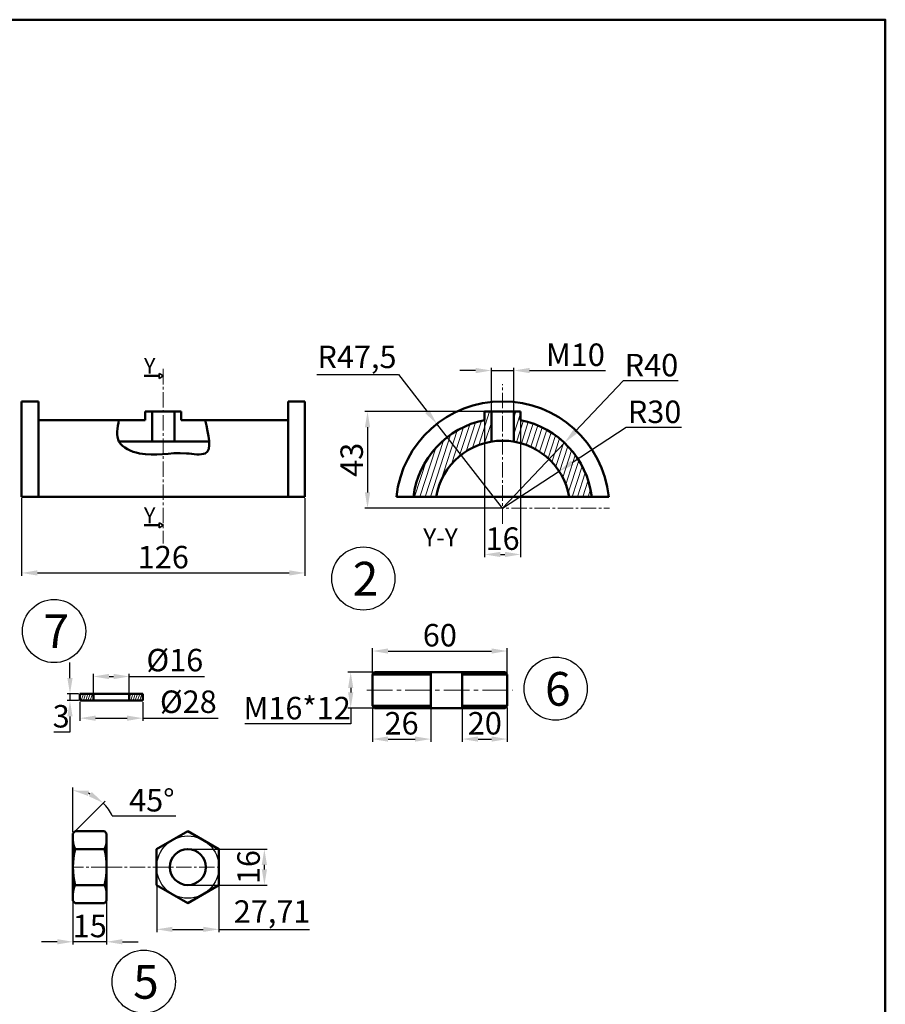
# Model space of a CAD drawing. Units: millimetres. Extents: x -68 to 1086, y -293 to 557.
# Tile 4 of 4: x 701 to 1086, y 119 to 557. Entities that reach past the tile are written whole.
import ezdxf

# ---------------------------------------------------------------- set-up
doc = ezdxf.new("R2010")
doc.units = ezdxf.units.MM
doc.header["$LTSCALE"] = 0.6
doc.linetypes.add('CENTER2', pattern=[28.575, 19.05, -3.175, 3.175, -3.175])
for name, color, linetype, lineweight in [('M-CNTR', 1, 'CENTER2', 18), ('M-DIMS', 2, 'Continuous', 25), ('M-HATC', 8, 'Continuous', 18), ('M-OUTL', 7, 'Continuous', 50), ('M-SECT', 6, 'Continuous', 35), ('M-SYMB', 4, 'Continuous', 25), ('M-TEXT', 3, 'Continuous', 25)]:
    doc.layers.add(name, color=color, linetype=linetype, lineweight=lineweight)
doc.styles.get("Standard").update_dxf_attribs({"font": 'arial.ttf'})
doc.dimstyles.new('ISO-25', dxfattribs={"dimtxt": 10, "dimasz": 7, "dimexe": 1.25, "dimexo": 0.625, "dimtad": 1, "dimtoh": 1, "dimtxsty": 'Standard', "dimcen": 2.5, "dimadec": 0, "dimazin": 0, "dimtfac": 1, "dimtmove": 0, "dimatfit": 3, "dimfxl": 1, "dimarcsym": 0})

# ---------------------------------------------------------------- blocks, each defined once
blk = doc.blocks.new('*D54')
at = {"layer": 'Defpoints', "color": 0, "ltscale": 0.6, "transparency": 16777216}
for p in [(701.62, 344.28), (827.62, 344.28), (827.62, 310.45)]:
    blk.add_point(p, dxfattribs=at)
at = {"layer": 'M-DIMS', "color": 0, "lineweight": -2, "ltscale": 0.6, "transparency": 16777216}
for p, q in [((701.62, 343.66), (701.62, 309.2)), ((827.62, 343.66), (827.62, 309.2)), ((708.62, 310.45), (820.62, 310.45))]:
    blk.add_line(p, q, dxfattribs=at)
at = {"layer": 'M-DIMS', "color": 0, "ltscale": 0.6, "transparency": 16777216}
for points in [[(708.62, 311.62), (708.62, 309.28), (701.62, 310.45)], [(820.62, 311.62), (820.62, 309.28), (827.62, 310.45)]]:
    blk.add_solid(points, dxfattribs=at)
at = {"layer": 'M-DIMS', "color": 0, "ltscale": 0.6, "transparency": 16777216, "insert": (764.62, 316.18), "char_height": 10, "attachment_point": 5}
blk.add_mtext('126', dxfattribs=at)
blk = doc.blocks.new('*D55')
at = {"layer": 'Defpoints', "color": 0, "ltscale": 0.6, "transparency": 16777216}
for p in [(940.63, 355.65), (915.49, 339.28)]:
    blk.add_point(p, dxfattribs=at)
at = {"layer": 'M-DIMS', "color": 0, "lineweight": -2, "ltscale": 0.6, "transparency": 16777216}
for p, q in [((970.51, 375.11), (946.5, 359.47)), ((995, 375.11), (970.51, 375.11)), ((915.49, 339.28), (940.63, 355.65))]:
    blk.add_line(p, q, dxfattribs=at)
at = {"layer": 'M-DIMS', "color": 0, "ltscale": 0.6, "transparency": 16777216}
blk.add_solid([(945.86, 360.45), (947.13, 358.5), (940.63, 355.65)], dxfattribs=at)
at = {"layer": 'M-DIMS', "color": 0, "ltscale": 0.6, "transparency": 16777216, "insert": (983.07, 380.84), "char_height": 10, "attachment_point": 5}
blk.add_mtext('R30', dxfattribs=at)
blk = doc.blocks.new('*D56')
at = {"layer": 'Defpoints', "color": 0, "ltscale": 0.6, "transparency": 16777216}
for p in [(943, 368.32), (915.49, 339.28)]:
    blk.add_point(p, dxfattribs=at)
at = {"layer": 'M-DIMS', "color": 0, "lineweight": -2, "ltscale": 0.6, "transparency": 16777216}
for p, q in [((969.12, 395.89), (947.82, 373.4)), ((993.61, 395.89), (969.12, 395.89)), ((915.49, 339.28), (943, 368.32))]:
    blk.add_line(p, q, dxfattribs=at)
at = {"layer": 'M-DIMS', "color": 0, "ltscale": 0.6, "transparency": 16777216}
blk.add_solid([(946.97, 374.21), (948.66, 372.6), (943, 368.32)], dxfattribs=at)
at = {"layer": 'M-DIMS', "color": 0, "ltscale": 0.6, "transparency": 16777216, "insert": (981.68, 401.62), "char_height": 10, "attachment_point": 5}
blk.add_mtext('R40', dxfattribs=at)
blk = doc.blocks.new('*D57')
at = {"layer": 'Defpoints', "color": 0, "ltscale": 0.6, "transparency": 16777216}
for p in [(886.28, 376.74), (915.49, 339.28)]:
    blk.add_point(p, dxfattribs=at)
at = {"layer": 'M-DIMS', "color": 0, "lineweight": -2, "ltscale": 0.6, "transparency": 16777216}
for p, q in [((832.92, 398.68), (869.17, 398.68)), ((869.17, 398.68), (881.97, 382.26)), ((915.49, 339.28), (886.28, 376.74))]:
    blk.add_line(p, q, dxfattribs=at)
at = {"layer": 'M-DIMS', "color": 0, "ltscale": 0.6, "transparency": 16777216}
blk.add_solid([(882.89, 382.98), (881.05, 381.54), (886.28, 376.74)], dxfattribs=at)
at = {"layer": 'M-DIMS', "color": 0, "ltscale": 0.6, "transparency": 16777216, "insert": (850.73, 405.29), "char_height": 10, "attachment_point": 5}
blk.add_mtext('R47,5', dxfattribs=at)
blk = doc.blocks.new('*D58')
at = {"layer": 'Defpoints', "color": 0, "ltscale": 0.6, "transparency": 16777216}
for p in [(907.49, 382.28), (923.49, 382.28), (923.49, 318.67)]:
    blk.add_point(p, dxfattribs=at)
at = {"layer": 'M-DIMS', "color": 0, "lineweight": -2, "ltscale": 0.6, "transparency": 16777216}
for p, q in [((907.49, 381.66), (907.49, 317.42)), ((923.49, 381.66), (923.49, 317.42)), ((914.49, 318.67), (916.49, 318.67))]:
    blk.add_line(p, q, dxfattribs=at)
at = {"layer": 'M-DIMS', "color": 0, "ltscale": 0.6, "transparency": 16777216}
for points in [[(914.49, 319.84), (914.49, 317.51), (907.49, 318.67)], [(916.49, 319.84), (916.49, 317.51), (923.49, 318.67)]]:
    blk.add_solid(points, dxfattribs=at)
at = {"layer": 'M-DIMS', "color": 0, "ltscale": 0.6, "transparency": 16777216, "insert": (915.49, 324.41), "char_height": 10, "attachment_point": 5}
blk.add_mtext('16', dxfattribs=at)
blk = doc.blocks.new('*D59')
at = {"layer": 'Defpoints', "color": 0, "ltscale": 0.6, "transparency": 16777216}
for p in [(920.49, 400.5), (910.49, 382.28), (920.49, 382.28)]:
    blk.add_point(p, dxfattribs=at)
at = {"layer": 'M-DIMS', "color": 0, "lineweight": -2, "ltscale": 0.6, "transparency": 16777216}
for p, q in [((903.49, 400.5), (896.49, 400.5)), ((910.49, 382.91), (910.49, 401.75)), ((910.49, 400.5), (920.49, 400.5)), ((920.49, 382.91), (920.49, 401.75)), ((927.49, 400.5), (961.21, 400.5))]:
    blk.add_line(p, q, dxfattribs=at)
at = {"layer": 'M-DIMS', "color": 0, "ltscale": 0.6, "transparency": 16777216}
for points in [[(903.49, 401.66), (903.49, 399.33), (910.49, 400.5)], [(927.49, 401.66), (927.49, 399.33), (920.49, 400.5)]]:
    blk.add_solid(points, dxfattribs=at)
at = {"layer": 'M-DIMS', "color": 0, "ltscale": 0.6, "transparency": 16777216, "insert": (947.85, 406.23), "char_height": 10, "attachment_point": 5}
blk.add_mtext('M10', dxfattribs=at)
blk = doc.blocks.new('*D60')
at = {"layer": 'Defpoints', "color": 0, "ltscale": 0.6, "transparency": 16777216}
for p in [(915.49, 382.28), (855.42, 339.28), (915.49, 339.28)]:
    blk.add_point(p, dxfattribs=at)
at = {"layer": 'M-DIMS', "color": 0, "lineweight": -2, "ltscale": 0.6, "transparency": 16777216}
for p, q in [((914.87, 382.28), (854.17, 382.28)), ((855.42, 375.28), (855.42, 346.28)), ((914.87, 339.28), (854.17, 339.28))]:
    blk.add_line(p, q, dxfattribs=at)
at = {"layer": 'M-DIMS', "color": 0, "ltscale": 0.6, "transparency": 16777216}
for points in [[(854.26, 375.28), (856.59, 375.28), (855.42, 382.28)], [(854.26, 346.28), (856.59, 346.28), (855.42, 339.28)]]:
    blk.add_solid(points, dxfattribs=at)
at = {"layer": 'M-DIMS', "color": 0, "ltscale": 0.6, "transparency": 16777216, "insert": (849.69, 360.78), "char_height": 10, "attachment_point": 5, "rotation": 90}
blk.add_mtext('43', dxfattribs=at)
blk = doc.blocks.new('*D61')
at = {"layer": 'Defpoints', "color": 0, "ltscale": 0.6, "transparency": 16777216}
for p in [(749.5, 264.36), (733.5, 256.64), (749.5, 256.64)]:
    blk.add_point(p, dxfattribs=at)
at = {"layer": 'M-DIMS', "color": 0, "lineweight": -2, "ltscale": 0.6, "transparency": 16777216}
for p, q in [((733.5, 257.26), (733.5, 265.61)), ((740.5, 264.36), (742.5, 264.36)), ((749.5, 257.26), (749.5, 265.61)), ((749.5, 264.36), (782.95, 264.36))]:
    blk.add_line(p, q, dxfattribs=at)
at = {"layer": 'M-DIMS', "color": 0, "ltscale": 0.6, "transparency": 16777216}
for points in [[(740.5, 265.53), (740.5, 263.19), (733.5, 264.36)], [(742.5, 265.53), (742.5, 263.19), (749.5, 264.36)]]:
    blk.add_solid(points, dxfattribs=at)
at = {"layer": 'M-DIMS', "color": 0, "ltscale": 0.6, "transparency": 16777216, "insert": (769.73, 270.37), "char_height": 10, "attachment_point": 5}
blk.add_mtext('%%C16', dxfattribs=at)
blk = doc.blocks.new('*D62')
at = {"layer": 'Defpoints', "color": 0, "ltscale": 0.6, "transparency": 16777216}
for p in [(727.5, 253.64), (755.5, 253.64), (755.5, 245.83)]:
    blk.add_point(p, dxfattribs=at)
at = {"layer": 'M-DIMS', "color": 0, "lineweight": -2, "ltscale": 0.6, "transparency": 16777216}
for p, q in [((727.5, 253.01), (727.5, 244.58)), ((755.5, 253.01), (755.5, 244.58)), ((734.5, 245.83), (748.5, 245.83)), ((755.5, 245.83), (788.98, 245.83))]:
    blk.add_line(p, q, dxfattribs=at)
at = {"layer": 'M-DIMS', "color": 0, "ltscale": 0.6, "transparency": 16777216}
for points in [[(734.5, 246.99), (734.5, 244.66), (727.5, 245.83)], [(748.5, 246.99), (748.5, 244.66), (755.5, 245.83)]]:
    blk.add_solid(points, dxfattribs=at)
at = {"layer": 'M-DIMS', "color": 0, "ltscale": 0.6, "transparency": 16777216, "insert": (775.74, 251.84), "char_height": 10, "attachment_point": 5}
blk.add_mtext('%%C28', dxfattribs=at)
blk = doc.blocks.new('*D63')
at = {"layer": 'Defpoints', "color": 0, "ltscale": 0.6, "transparency": 16777216}
for p in [(727.5, 256.64), (723.1, 253.64), (727.5, 253.64)]:
    blk.add_point(p, dxfattribs=at)
at = {"layer": 'M-DIMS', "color": 0, "lineweight": -2, "ltscale": 0.6, "transparency": 16777216}
for p, q in [((723.1, 263.64), (723.1, 270.64)), ((726.88, 256.64), (721.85, 256.64)), ((723.1, 256.64), (723.1, 253.64)), ((726.88, 253.64), (721.85, 253.64)), ((723.1, 246.64), (723.1, 239.64)), ((723.1, 239.64), (715.93, 239.64))]:
    blk.add_line(p, q, dxfattribs=at)
at = {"layer": 'M-DIMS', "color": 0, "ltscale": 0.6, "transparency": 16777216}
for points in [[(721.94, 263.64), (724.27, 263.64), (723.1, 256.64)], [(721.94, 246.64), (724.27, 246.64), (723.1, 253.64)]]:
    blk.add_solid(points, dxfattribs=at)
at = {"layer": 'M-DIMS', "color": 0, "ltscale": 0.6, "transparency": 16777216, "insert": (719.2, 245.37), "char_height": 10, "attachment_point": 5}
blk.add_mtext('3', dxfattribs=at)
blk = doc.blocks.new('*D64')
at = {"layer": 'Defpoints', "color": 0, "ltscale": 0.6, "transparency": 16777216}
for p in [(724.42, 166.01), (739.42, 166.01), (724.42, 146.34)]:
    blk.add_point(p, dxfattribs=at)
at = {"layer": 'M-DIMS', "color": 0, "lineweight": -2, "ltscale": 0.6, "transparency": 16777216}
for p, q in [((724.42, 165.39), (724.42, 145.09)), ((739.42, 165.39), (739.42, 145.09)), ((717.42, 146.34), (710.42, 146.34)), ((739.42, 146.34), (724.42, 146.34)), ((746.42, 146.34), (753.42, 146.34))]:
    blk.add_line(p, q, dxfattribs=at)
at = {"layer": 'M-DIMS', "color": 0, "ltscale": 0.6, "transparency": 16777216}
for points in [[(717.42, 147.51), (717.42, 145.17), (724.42, 146.34)], [(746.42, 147.51), (746.42, 145.17), (739.42, 146.34)]]:
    blk.add_solid(points, dxfattribs=at)
at = {"layer": 'M-DIMS', "color": 0, "ltscale": 0.6, "transparency": 16777216, "insert": (731.92, 152.07), "char_height": 10, "attachment_point": 5}
blk.add_mtext('15', dxfattribs=at)
blk = doc.blocks.new('*D65')
at = {"layer": 'Defpoints', "color": 0, "ltscale": 0.6, "transparency": 16777216}
for p in [(729.37, 213.02), (724.42, 194.57), (724.42, 194.57), (725.42, 195.57), (724.42, 164.57)]:
    blk.add_point(p, dxfattribs=at)
at = {"layer": 'M-DIMS', "color": 0, "lineweight": -2, "ltscale": 0.6, "transparency": 16777216}
for p, q in [((724.42, 195.2), (724.42, 214.93)), ((725.87, 196.02), (738.81, 208.96)), ((741.89, 202.31), (770.16, 202.31))]:
    blk.add_line(p, q, dxfattribs=at)
for start, end in [(66.1169, 68.8831), (23.8831, 45)]:
    blk.add_arc((724.42, 194.57), 19.1, start, end, dxfattribs=at)
at = {"layer": 'M-DIMS', "color": 0, "ltscale": 0.6, "transparency": 16777216}
for points in [[(731.09, 211.25), (731.52, 213.54), (724.42, 213.68)], [(732.82, 213), (731.5, 211.08), (737.93, 208.08)]]:
    blk.add_solid(points, dxfattribs=at)
at = {"layer": 'M-DIMS', "color": 0, "ltscale": 0.6, "transparency": 16777216, "insert": (759.52, 208.02), "char_height": 10, "attachment_point": 5}
blk.add_mtext('45°', dxfattribs=at)
blk = doc.blocks.new('*D66')
at = {"layer": 'Defpoints', "color": 0, "ltscale": 0.6, "transparency": 16777216}
for p in [(761.66, 171.57), (789.37, 171.57), (789.37, 151.87)]:
    blk.add_point(p, dxfattribs=at)
at = {"layer": 'M-DIMS', "color": 0, "lineweight": -2, "ltscale": 0.6, "transparency": 16777216}
for p, q in [((761.66, 170.95), (761.66, 150.62)), ((789.37, 170.95), (789.37, 150.62)), ((768.66, 151.87), (782.37, 151.87)), ((789.37, 151.87), (829.6, 151.87))]:
    blk.add_line(p, q, dxfattribs=at)
at = {"layer": 'M-DIMS', "color": 0, "ltscale": 0.6, "transparency": 16777216}
for points in [[(768.66, 153.03), (768.66, 150.7), (761.66, 151.87)], [(782.37, 153.03), (782.37, 150.7), (789.37, 151.87)]]:
    blk.add_solid(points, dxfattribs=at)
at = {"layer": 'M-DIMS', "color": 0, "ltscale": 0.6, "transparency": 16777216, "insert": (812.99, 158.5), "char_height": 10, "attachment_point": 5}
blk.add_mtext('27,71', dxfattribs=at)
blk = doc.blocks.new('*D67')
at = {"layer": 'Defpoints', "color": 0, "ltscale": 0.6, "transparency": 16777216}
for p in [(775.51, 187.57), (809.56, 187.57), (775.51, 171.57)]:
    blk.add_point(p, dxfattribs=at)
at = {"layer": 'M-DIMS', "color": 0, "lineweight": -2, "ltscale": 0.6, "transparency": 16777216}
for p, q in [((776.14, 187.57), (810.81, 187.57)), ((809.56, 178.57), (809.56, 180.57)), ((776.14, 171.57), (810.81, 171.57))]:
    blk.add_line(p, q, dxfattribs=at)
at = {"layer": 'M-DIMS', "color": 0, "ltscale": 0.6, "transparency": 16777216}
for points in [[(808.39, 180.57), (810.72, 180.57), (809.56, 187.57)], [(808.39, 178.57), (810.72, 178.57), (809.56, 171.57)]]:
    blk.add_solid(points, dxfattribs=at)
at = {"layer": 'M-DIMS', "color": 0, "ltscale": 0.6, "transparency": 16777216, "insert": (803.83, 179.57), "char_height": 10, "attachment_point": 5, "rotation": 90}
blk.add_mtext('16', dxfattribs=at)
blk = doc.blocks.new('*U71')
at = {"layer": 'M-CNTR', "color": 0, "transparency": 16777216}
blk.add_line((-32.5, 0), (32.5, 0), dxfattribs=at)
blk = doc.blocks.new('*D72')
at = {"layer": 'Defpoints', "color": 0, "ltscale": 0.6, "transparency": 16777216}
for p in [(917.58, 275.7), (857.58, 262.16), (917.58, 262.16)]:
    blk.add_point(p, dxfattribs=at)
at = {"layer": 'M-DIMS', "color": 0, "lineweight": -2, "ltscale": 0.6, "transparency": 16777216}
for p, q in [((857.58, 262.78), (857.58, 276.95)), ((917.58, 262.78), (917.58, 276.95)), ((864.58, 275.7), (910.58, 275.7))]:
    blk.add_line(p, q, dxfattribs=at)
at = {"layer": 'M-DIMS', "color": 0, "ltscale": 0.6, "transparency": 16777216}
for points in [[(864.58, 276.87), (864.58, 274.54), (857.58, 275.7)], [(910.58, 276.87), (910.58, 274.54), (917.58, 275.7)]]:
    blk.add_solid(points, dxfattribs=at)
at = {"layer": 'M-DIMS', "color": 0, "ltscale": 0.6, "transparency": 16777216, "insert": (887.58, 281.43), "char_height": 10, "attachment_point": 5}
blk.add_mtext('60', dxfattribs=at)
blk = doc.blocks.new('*D73')
at = {"layer": 'Defpoints', "color": 0, "ltscale": 0.6, "transparency": 16777216}
for p in [(857.58, 251.27), (883.58, 251.27), (883.58, 236.53)]:
    blk.add_point(p, dxfattribs=at)
at = {"layer": 'M-DIMS', "color": 0, "lineweight": -2, "ltscale": 0.6, "transparency": 16777216}
for p, q in [((857.58, 250.64), (857.58, 235.28)), ((883.58, 250.64), (883.58, 235.28)), ((864.58, 236.53), (876.58, 236.53))]:
    blk.add_line(p, q, dxfattribs=at)
at = {"layer": 'M-DIMS', "color": 0, "ltscale": 0.6, "transparency": 16777216}
for points in [[(864.58, 237.7), (864.58, 235.37), (857.58, 236.53)], [(876.58, 237.7), (876.58, 235.37), (883.58, 236.53)]]:
    blk.add_solid(points, dxfattribs=at)
at = {"layer": 'M-DIMS', "color": 0, "ltscale": 0.6, "transparency": 16777216, "insert": (870.58, 242.26), "char_height": 10, "attachment_point": 5}
blk.add_mtext('26', dxfattribs=at)
blk = doc.blocks.new('*D74')
at = {"layer": 'Defpoints', "color": 0, "ltscale": 0.6, "transparency": 16777216}
for p in [(897.58, 251.27), (917.58, 251.27), (917.58, 236.53)]:
    blk.add_point(p, dxfattribs=at)
at = {"layer": 'M-DIMS', "color": 0, "lineweight": -2, "ltscale": 0.6, "transparency": 16777216}
for p, q in [((897.58, 250.64), (897.58, 235.28)), ((917.58, 250.64), (917.58, 235.28)), ((904.58, 236.53), (910.58, 236.53))]:
    blk.add_line(p, q, dxfattribs=at)
at = {"layer": 'M-DIMS', "color": 0, "ltscale": 0.6, "transparency": 16777216}
for points in [[(904.58, 237.7), (904.58, 235.37), (897.58, 236.53)], [(910.58, 237.7), (910.58, 235.37), (917.58, 236.53)]]:
    blk.add_solid(points, dxfattribs=at)
at = {"layer": 'M-DIMS', "color": 0, "ltscale": 0.6, "transparency": 16777216, "insert": (907.58, 242.26), "char_height": 10, "attachment_point": 5}
blk.add_mtext('20', dxfattribs=at)
blk = doc.blocks.new('*D75')
at = {"layer": 'Defpoints', "color": 0, "ltscale": 0.6, "transparency": 16777216}
for p in [(858.58, 266.27), (847.94, 250.27), (858.58, 250.27)]:
    blk.add_point(p, dxfattribs=at)
at = {"layer": 'M-DIMS', "color": 0, "lineweight": -2, "ltscale": 0.6, "transparency": 16777216}
for p, q in [((857.95, 266.27), (846.69, 266.27)), ((847.94, 259.27), (847.94, 257.27)), ((857.95, 250.27), (846.69, 250.27)), ((847.94, 250.27), (847.94, 243.27)), ((847.94, 243.27), (800.93, 243.27))]:
    blk.add_line(p, q, dxfattribs=at)
at = {"layer": 'M-DIMS', "color": 0, "ltscale": 0.6, "transparency": 16777216}
for points in [[(846.77, 259.27), (849.1, 259.27), (847.94, 266.27)], [(846.77, 257.27), (849.1, 257.27), (847.94, 250.27)]]:
    blk.add_solid(points, dxfattribs=at)
at = {"layer": 'M-DIMS', "color": 0, "ltscale": 0.6, "transparency": 16777216, "insert": (824.12, 249), "char_height": 10, "attachment_point": 5}
blk.add_mtext('M16*12', dxfattribs=at)
blk = doc.blocks.new('NUT-SIDE')
at = {"ltscale": 0.6}
for p, q in [((1, 32), (0, 31)), ((0, 1), (0, 31)), ((1, 32), (14, 32)), ((15, 31), (14, 32)), ((15, 31), (15, 1)), ((14, 24), (1, 24)), ((14, 8), (1, 8)), ((0, 1), (1, 0)), ((14, 0), (1, 0)), ((15, 1), (14, 0))]:
    blk.add_line(p, q, dxfattribs=at)
for centre, radius, start, end in [((8.5, 28), 8.5, 180, 208.0725), ((6.5, 28), 8.5, 331.9275, 0), ((32.5, 16), 32.5, 165.75, 194.25), ((-17.5, 16), 32.5, 345.75, 14.25), ((8.5, 4), 8.5, 151.9275, 180), ((6.5, 4), 8.5, 0, 28.0725)]:
    blk.add_arc(centre, radius, start, end, dxfattribs=at)
blk = doc.blocks.new('WASHER-SIDE')
at = {"ltscale": 0.6}
for p, q in [((0, 3), (28, 3)), ((0, 0), (0, 3)), ((28, 0), (0, 0)), ((28, 3), (28, 0))]:
    blk.add_line(p, q, dxfattribs=at)
blk = doc.blocks.new('SECT-ARROW')
at = {"ltscale": 0.6}
for p, q in [((1.92, 1.11), (0, 2.22)), ((0, 2.22), (0, 0)), ((1.92, 1.11), (0, 0))]:
    blk.add_line(p, q, dxfattribs=at)

msp = doc.modelspace()

# ---------------------------------------------------------------- hatches: boundary and pattern name
at = {"layer": 'M-HATC', "ltscale": 0.6}
h = msp.add_hatch(dxfattribs=at)
h.set_pattern_fill('ANSI31', color=256, scale=0.7, angle=27)
h.set_pattern_definition([(72, (166.6146, 303.1702), (-2.113723, 0.68679), [])])
h.paths.add_polyline_path([(910.492, 368.865), (910.492, 382.284), (907.492, 382.284), (907.492, 378.476, 0.321461), (875.805, 344.284), (885.911, 344.284, -0.3191977)])
h.paths.add_polyline_path([(945.072, 344.284), (955.178, 344.284, 0.321461), (923.492, 378.476), (923.492, 382.284), (920.492, 382.284), (920.492, 368.865, -0.3191977)])
h = msp.add_hatch(dxfattribs=at)
h.set_pattern_fill('ANSI31', color=256, scale=0.3, angle=27)
h.set_pattern_definition([(72, (-83.0523, 25.7486), (-0.9058813, 0.2943387), [])])
h.paths.add_polyline_path([(749.502, 256.636), (749.502, 253.636), (755.502, 253.636), (755.502, 256.636)])
h.paths.add_polyline_path([(733.502, 253.636), (733.502, 256.636), (727.502, 256.636), (727.502, 253.636)])

# ---------------------------------------------------------------- linework, layer by layer
at = {"layer": 'M-CNTR', "ltscale": 0.6}
for p, q in [((764.618, 401.189), (764.618, 323.467)), ((915.492, 332.296), (915.492, 394.447)), ((867.992, 339.284), (962.992, 339.284)), ((739.424, 179.574), (724.424, 179.574)), ((739.424, 179.574), (790.587, 179.574))]:
    msp.add_line(p, q, dxfattribs=at)
at = {"layer": 'M-OUTL', "ltscale": 0.6}
for p, q in [((762.886, 398.105), (756.143, 398.105)), ((701.618, 344.284), (701.618, 386.784)), ((701.618, 386.784), (709.118, 386.784)), ((709.118, 386.784), (709.118, 344.284)), ((820.118, 386.784), (820.118, 344.284)), ((820.118, 386.784), (827.618, 386.784)), ((827.618, 344.284), (827.618, 386.784)), ((772.618, 382.284), (756.618, 382.284)), ((756.618, 382.284), (756.618, 378.476)), ((759.618, 382.284), (759.618, 368.865)), ((769.618, 382.284), (769.618, 368.865)), ((772.618, 382.284), (772.618, 378.476)), ((907.492, 378.476), (907.492, 382.284)), ((907.492, 382.284), (923.492, 382.284)), ((910.492, 368.865), (910.492, 382.284)), ((920.492, 368.865), (920.492, 382.284)), ((923.492, 378.476), (923.492, 382.284)), ((756.618, 378.476), (709.118, 378.476)), ((820.118, 378.476), (772.618, 378.476)), ((785.053, 368.865), (744.907, 368.865)), ((827.618, 344.284), (701.618, 344.284)), ((868.255, 344.284), (962.728, 344.284)), ((762.886, 331.637), (756.143, 331.637)), ((858.577, 266.27), (857.577, 265.27)), ((857.577, 251.27), (857.577, 265.27)), ((857.577, 265.27), (883.577, 265.27)), ((858.577, 266.27), (916.577, 266.27)), ((883.577, 250.27), (883.577, 266.27)), ((897.577, 266.27), (897.577, 250.27)), ((917.577, 265.27), (897.577, 265.27)), ((916.577, 266.27), (917.577, 265.27)), ((917.577, 265.27), (917.577, 251.27)), ((733.502, 253.636), (733.502, 256.636)), ((749.502, 256.636), (749.502, 253.636)), ((857.577, 251.27), (858.577, 250.27)), ((857.577, 251.27), (883.577, 251.27)), ((916.577, 250.27), (858.577, 250.27)), ((917.577, 251.27), (897.577, 251.27)), ((917.577, 251.27), (916.577, 250.27))]:
    msp.add_line(p, q, dxfattribs=at)
for points in [[(-68.392, 556.589), (1085.677, 556.589), (1085.677, -292.72), (-68.392, -292.72)], [(775.512, 195.574), (761.656, 187.574), (761.656, 171.574), (775.512, 163.574), (789.369, 171.574), (789.369, 187.574)]]:
    msp.add_lwpolyline(points, close=True, dxfattribs=at)
msp.add_circle((775.512, 179.574), 8, dxfattribs=at)
for radius, start, end in [(47.5, 6.04233, 173.95767), (40, 101.53696, 172.81924), (40, 7.18076, 78.46304), (30, 9.59407, 170.40593)]:
    msp.add_arc((915.492, 339.284), radius, start, end, dxfattribs=at)
msp.add_open_spline([(744.907, 378.476), (744.219, 374.956), (742.781, 367.601), (758.245, 361.048), (769.461, 365.066), (787.388, 361.544), (784.827, 371.858), (783.183, 378.476)], degree=3, knots=[0, 0, 0, 0, 9.611437, 20.0803576, 40.9991508, 49.2899789, 64.1358762, 64.1358762, 64.1358762, 64.1358762], dxfattribs=at)
at = {"layer": 'M-SYMB', "ltscale": 0.6}
for centre, radius in [((853.555, 307.967), 14.053), ((716.05, 284.583), 14.053), ((939.076, 258.962), 14.053), ((775.512, 179.574), 13.856), ((755.919, 128.606), 14.053)]:
    msp.add_circle(centre, radius, dxfattribs=at)

# ---------------------------------------------------------------- block references
at = {"layer": 'M-CNTR'}
msp.add_blockref('*U71', (887.577, 258.27), dxfattribs=at)
at = {"layer": 'M-OUTL'}
for name, p in [('WASHER-SIDE', (727.502, 253.636)), ('NUT-SIDE', (724.424, 163.574))]:
    msp.add_blockref(name, p, dxfattribs=at)
at = {"layer": 'M-SECT'}
for p in [(762.824, 396.996), (762.824, 330.529)]:
    msp.add_blockref('SECT-ARROW', p, dxfattribs=at)

# ---------------------------------------------------------------- texts
at = {"layer": 'M-TEXT', "ltscale": 0.6, "attachment_point": 1}
for s, width, insert, char_height in [('Y', 4.24472, (756.023, 406.049), 7), ('Y', 4.24472, (756.023, 339.582), 7), ('Y-Y', 23.26032, (880.17, 330.264), 8), ('2', 15, (848.849, 315.374), 15), ('7', 15, (711.344, 291.99), 15), ('6', 15, (934.37, 266.369), 15), ('5', 15, (751.213, 136.013), 15)]:
    msp.add_mtext_dynamic_manual_height_columns(s, width=width, gutter_width=12.5, heights=[0], dxfattribs=dict(at, insert=insert, char_height=char_height))

# ---------------------------------------------------------------- dimensions: what is measured, and where the dimension line sits
at = {"layer": 'M-DIMS', "ltscale": 0.6}
for mpoint, picture, middle in [((886.279, 376.739), '*D57', (850.732, 398.679)), ((943.002, 368.322), '*D56', (981.675, 395.889)), ((940.632, 355.654), '*D55', (983.068, 375.11))]:
    dim = msp.add_radius_dim(center=(915.492, 339.284), mpoint=mpoint, dimstyle='ISO-25', override={"dimclrd": 0, "dimclre": 0, "dimclrt": 0}, dxfattribs=at)
    dim.commit()
    dim.dimension.update_dxf_attribs({"geometry": picture, "text_midpoint": middle, "dimtype": 164})
for base, p1, p2, text, picture, middle in [((920.492, 400.495), (910.492, 382.284), (920.492, 382.284), 'M<>', '*D59', (947.852, 406.226)), ((749.502, 264.361), (733.502, 256.636), (749.502, 256.636), '%%C<>', '*D61', (769.726, 270.371))]:
    dim = msp.add_linear_dim(base=base, p1=p1, p2=p2, text=text, dimstyle='ISO-25', override={"dimclrd": 0, "dimclre": 0, "dimclrt": 0}, dxfattribs=at)
    dim.commit()
    dim.dimension.update_dxf_attribs({"geometry": picture, "text_midpoint": middle})
for base, p1, p2, picture, middle in [((855.424, 339.284), (915.492, 382.284), (915.492, 339.284), '*D60', (849.69, 360.784)), ((723.104, 253.636), (727.502, 256.636), (727.502, 253.636), '*D63', (719.205, 245.37)), ((809.557, 187.574), (775.512, 171.574), (775.512, 187.574), '*D67', (803.826, 179.574))]:
    dim = msp.add_linear_dim(base=base, p1=p1, p2=p2, angle=90, dimstyle='ISO-25', override={"dimclrd": 0, "dimclre": 0, "dimclrt": 0}, dxfattribs=at)
    dim.commit()
    dim.dimension.update_dxf_attribs({"geometry": picture, "text_midpoint": middle})
for base, p1, p2, picture, middle in [((923.492, 318.674), (907.492, 382.284), (923.492, 382.284), '*D58', (915.492, 324.405)), ((827.618, 310.45), (701.618, 344.284), (827.618, 344.284), '*D54', (764.618, 316.181)), ((917.577, 275.702), (857.577, 262.155), (917.577, 262.155), '*D72', (887.577, 281.433)), ((883.577, 236.533), (857.577, 251.27), (883.577, 251.27), '*D73', (870.577, 242.264)), ((917.577, 236.533), (897.577, 251.27), (917.577, 251.27), '*D74', (907.577, 242.264)), ((789.369, 151.867), (761.656, 171.574), (789.369, 171.574), '*D66', (812.986, 158.501)), ((724.424, 146.339), (739.424, 166.014), (724.424, 166.014), '*D64', (731.924, 152.069))]:
    dim = msp.add_linear_dim(base=base, p1=p1, p2=p2, dimstyle='ISO-25', override={"dimclrd": 0, "dimclre": 0, "dimclrt": 0}, dxfattribs=at)
    dim.commit()
    dim.dimension.update_dxf_attribs({"geometry": picture, "text_midpoint": middle})
dim = msp.add_linear_dim(base=(847.937, 250.27), p1=(858.577, 266.27), p2=(858.577, 250.27), angle=90, text='M<>*12', dimstyle='ISO-25', override={"dimclrd": 0, "dimclre": 0, "dimclrt": 0}, dxfattribs=at)
dim.commit()
dim.dimension.update_dxf_attribs({"geometry": '*D75', "text_midpoint": (824.123, 249)})
dim = msp.add_linear_dim(base=(755.502, 245.828), p1=(727.502, 253.636), p2=(755.502, 253.636), text='%%C<>', dimstyle='ISO-25', override={"dimclrd": 0, "dimclre": 0, "dimclrt": 0}, dxfattribs=at)
dim.commit()
dim.dimension.update_dxf_attribs({"geometry": '*D62', "text_midpoint": (775.74, 245.828), "dimtype": 160})
dim = msp.add_angular_dim_2l(base=(729.368, 213.024), line1=((725.424, 195.574), (724.424, 194.574)), line2=((724.424, 164.574), (724.424, 194.574)), dimstyle='ISO-25', override={"dimclrd": 0, "dimclre": 0, "dimclrt": 0}, dxfattribs=at)
dim.commit()
dim.dimension.update_dxf_attribs({"geometry": '*D65', "text_midpoint": (759.524, 208.018)})

doc.saveas('drawing.dxf')
